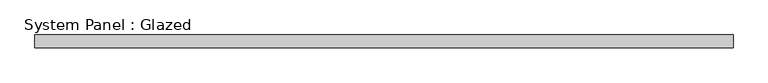
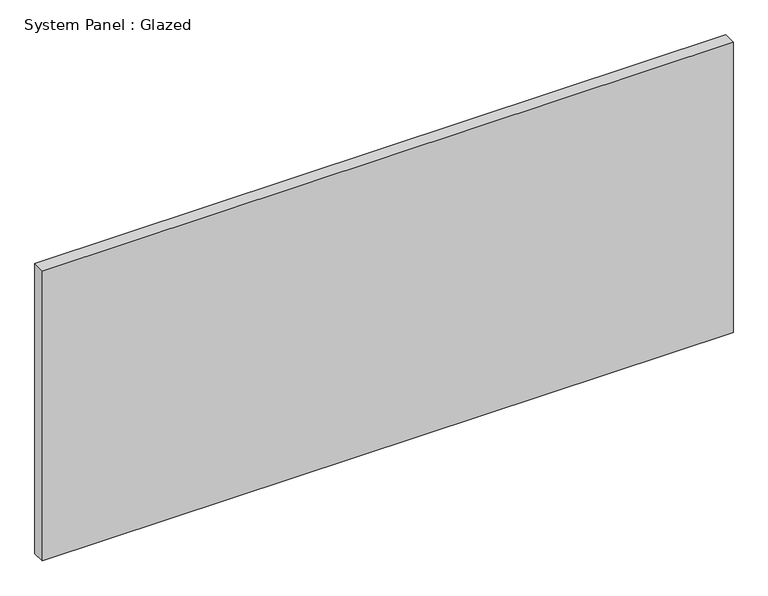
"""IFC4 building model written with IfcOpenShell, lengths in millimetres: plate geometry, System Panel : Glazed."""

from ifc_helpers import new_model, si_unit, origin, origin_with_axes, place, context, project, spatial, polyline, outline, extrude, source, transform, mapped, element, save


def system_panel_glazed_6115a09f(model_context):
    return source(origin(), model_context, "Body", "SweptSolid", [
        extrude(outline(polyline([(675.0, 24.5), (-675.0, 24.5), (-675.0, 49.5), (675.0, 49.5), (675.0, 24.5)])), origin_with_axes(), (0.0, 0.0, 1.0), 600.0),
    ])


if __name__ == "__main__":
    model = new_model("IFC4")
    model_context = context("Model", 3, world=origin())
    ifc_project = project(units=[si_unit("LENGTHUNIT", "METRE", prefix="MILLI")], contexts=[model_context])
    site = spatial("IfcSite", under=ifc_project)
    building = spatial("IfcBuilding", under=site)
    placement = place(None, origin())
    system_panel_glazed_shape = system_panel_glazed_6115a09f(model_context)
    element("IfcPlate", 1, ObjectType="System Panel : Glazed", at=placement, inside=building, context=model_context, shape_type="MappedRepresentation", body=[
        mapped(system_panel_glazed_shape, transform((0.0, 0.0, 0.0), x_axis=(1.0, 0.0, 0.0), y_axis=(0.0, 1.0, 0.0), z_axis=(0.0, 0.0, 1.0))),
    ])
    save(model, "model.ifc")

# Revit data of these elements
# Type "System Panel : Glazed"
#   Keynote = "H11"
#   Construction Type Id = "GSP4R"
#   Analytic Construction = "1/8 in Pilkington single glazing"
#   Visual Light Transmittance = 0.9
#   Solar Heat Gain Coefficient = 0.86
#   Heat Transfer Coefficient (U) = 6.7069 W/(m²·K)
#   Define Thermal Properties by = 1
# Element 1 (IfcPlate, "System Panel : Glazed")
#   Materials on its faces: "Glass"
# Materials
#   "Glass": class "Glass", colour RGB 0 128 192, transparency 0.9, Description = "Soda Lime Glass", Cost = 0
